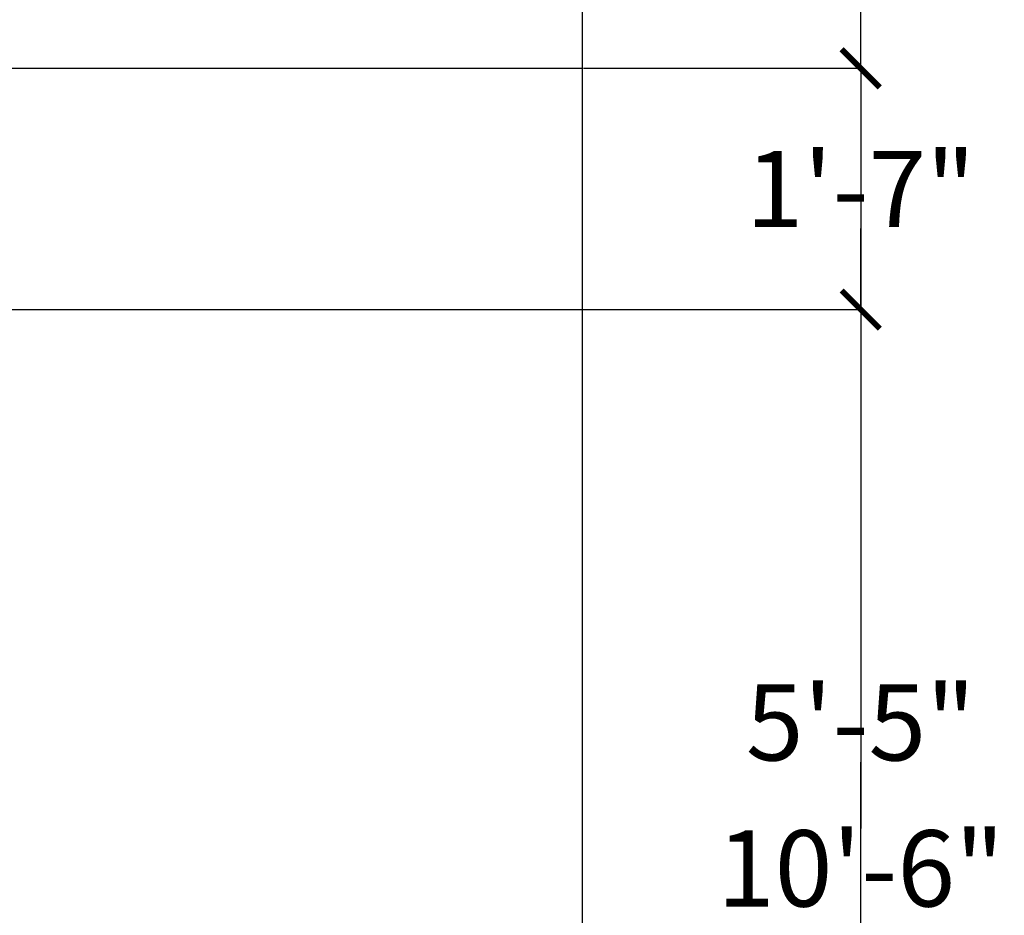
# Model space of a CAD drawing. Units: inches. Extents: x 2278 to 7495, y -71 to 1198.
# Tile 37 of 44: x 5101 to 5179, y 178 to 248. Entities that reach past the tile are written whole.
import ezdxf

# ---------------------------------------------------------------- set-up
doc = ezdxf.new("R2010")
doc.units = ezdxf.units.IN
doc.header["$MEASUREMENT"] = 0
doc.layers.add('A-ANNO-DIMS', color=2, linetype='Continuous', lineweight=18)
doc.layers.add('A-ELEV', color=7, linetype='Continuous', lineweight=25)
doc.styles.get("Standard").update_dxf_attribs({"font": 'arial.ttf'})
doc.dimstyles.get("Standard").update_dxf_attribs({"dimtxt": 6, "dimasz": 3, "dimexe": 0.18, "dimexo": 0.0625, "dimgap": 0.09, "dimtad": 0, "dimtih": 1, "dimtoh": 1, "dimdec": 0, "dimzin": 0, "dimdsep": 46, "dimlunit": 3, "dimtxsty": 'Standard', "dimblk": 'ARCHTICK', "dimcen": 0.09, "dimadec": 0, "dimazin": 0, "dimtfac": 1, "dimtdec": 0, "dimtofl": 0, "dimtmove": 0, "dimatfit": 3, "dimfxl": 1, "dimtolj": 1, "dimtzin": 0, "dimarcsym": 0})

# ---------------------------------------------------------------- blocks, each defined once
blk = doc.blocks.new('_ArchTick')
at = {"color": 0, "linetype": 'ByBlock', "const_width": 0.15}
blk.add_lwpolyline([(-0.5, -0.5), (0.5, 0.5)], dxfattribs=at)
blk = doc.blocks.new('*D123')
at = {"layer": 'A-ANNO-DIMS', "color": 0, "lineweight": -2, "transparency": 16777216}
for p, q in [((4736.95, 340.157), (4736.95, -23.427)), ((5145.676, -1.81), (5145.676, -23.427)), ((4736.95, -23.247), (4923.929, -23.247)), ((5145.676, -23.247), (4958.697, -23.247))]:
    blk.add_line(p, q, dxfattribs=at)
at = {"layer": 'Defpoints', "color": 0, "transparency": 16777216}
for p in [(4736.95, 340.219), (5145.676, -1.747), (5145.676, -23.247)]:
    blk.add_point(p, dxfattribs=at)
at = {"layer": 'A-ANNO-DIMS', "color": 0, "lineweight": -2, "transparency": 16777216, "xscale": 3, "yscale": 3, "zscale": 3, "rotation": 180}
blk.add_blockref('_ArchTick', (4736.95, -23.247), dxfattribs=at)
at = {"layer": 'A-ANNO-DIMS', "color": 0, "lineweight": -2, "transparency": 16777216, "xscale": 3, "yscale": 3, "zscale": 3}
blk.add_blockref('_ArchTick', (5145.676, -23.247), dxfattribs=at)
at = {"layer": 'A-ANNO-DIMS', "color": 0, "transparency": 16777216, "insert": (4941.313, -23.247), "char_height": 6, "attachment_point": 5}
blk.add_mtext('\\A1;34\'-0 1/2"', dxfattribs=at)
blk = doc.blocks.new('*D131')
at = {"layer": 'A-ANNO-DIMS', "color": 0, "lineweight": -2, "transparency": 16777216}
for p, q in [((5096.176, 99.315), (5096.176, 361.899)), ((5096.176, 361.719), (5105.75, 361.719)), ((5145.676, 361.719), (5136.102, 361.719)), ((5145.676, 118.315), (5145.676, 361.899))]:
    blk.add_line(p, q, dxfattribs=at)
at = {"layer": 'Defpoints', "color": 0, "transparency": 16777216}
for p in [(5145.676, 361.719), (5145.676, 118.253), (5096.176, 99.253)]:
    blk.add_point(p, dxfattribs=at)
at = {"layer": 'A-ANNO-DIMS', "color": 0, "lineweight": -2, "transparency": 16777216, "xscale": 3, "yscale": 3, "zscale": 3, "rotation": 180}
blk.add_blockref('_ArchTick', (5096.176, 361.719), dxfattribs=at)
at = {"layer": 'A-ANNO-DIMS', "color": 0, "lineweight": -2, "transparency": 16777216, "xscale": 3, "yscale": 3, "zscale": 3}
blk.add_blockref('_ArchTick', (5145.676, 361.719), dxfattribs=at)
at = {"layer": 'A-ANNO-DIMS', "color": 0, "transparency": 16777216, "insert": (5120.926, 361.719), "char_height": 6, "attachment_point": 5}
blk.add_mtext('\\A1;4\'-1 1/2"', dxfattribs=at)
blk = doc.blocks.new('*D140')
at = {"layer": 'A-ANNO-DIMS', "color": 0, "lineweight": -2, "transparency": 16777216}
for p, q in [((5096.239, 225.253), (5167.754, 225.253)), ((5167.574, 225.253), (5167.574, 195.894)), ((5167.574, 160.253), (5167.574, 189.612)), ((5092.239, 160.253), (5167.754, 160.253))]:
    blk.add_line(p, q, dxfattribs=at)
at = {"layer": 'Defpoints', "color": 0, "transparency": 16777216}
for p in [(5096.176, 225.253), (5167.574, 225.253), (5092.176, 160.253)]:
    blk.add_point(p, dxfattribs=at)
at = {"layer": 'A-ANNO-DIMS', "color": 0, "lineweight": -2, "transparency": 16777216, "xscale": 3, "yscale": 3, "zscale": 3}
for p, rotation in [((5167.574, 225.253), 90), ((5167.574, 160.253), 270)]:
    blk.add_blockref('_ArchTick', p, dxfattribs=dict(at, rotation=rotation))
at = {"layer": 'A-ANNO-DIMS', "color": 0, "transparency": 16777216, "insert": (5167.574, 192.753), "char_height": 6, "attachment_point": 5}
blk.add_mtext('\\A1;5\'-5"', dxfattribs=at)
blk = doc.blocks.new('*D141')
at = {"layer": 'A-ANNO-DIMS', "color": 0, "lineweight": -2, "transparency": 16777216}
for p, q in [((5145.739, 244.253), (5167.754, 244.253)), ((5167.574, 244.253), (5167.574, 237.855)), ((5167.574, 225.253), (5167.574, 231.651)), ((5096.239, 225.253), (5167.754, 225.253))]:
    blk.add_line(p, q, dxfattribs=at)
at = {"layer": 'Defpoints', "color": 0, "transparency": 16777216}
for p in [(5145.676, 244.253), (5167.574, 244.253), (5096.176, 225.253)]:
    blk.add_point(p, dxfattribs=at)
at = {"layer": 'A-ANNO-DIMS', "color": 0, "lineweight": -2, "transparency": 16777216, "xscale": 3, "yscale": 3, "zscale": 3}
for p, rotation in [((5167.574, 244.253), 90), ((5167.574, 225.253), 270)]:
    blk.add_blockref('_ArchTick', p, dxfattribs=dict(at, rotation=rotation))
at = {"layer": 'A-ANNO-DIMS', "color": 0, "transparency": 16777216, "insert": (5167.574, 234.753), "char_height": 6, "attachment_point": 5}
blk.add_mtext('\\A1;1\'-7"', dxfattribs=at)
blk = doc.blocks.new('*D142')
at = {"layer": 'A-ANNO-DIMS', "color": 0, "lineweight": -2, "transparency": 16777216}
for p, q in [((5143.335, 286.303), (5167.754, 286.303)), ((5167.574, 286.303), (5167.574, 268.433)), ((5167.574, 244.253), (5167.574, 262.122)), ((5145.739, 244.253), (5167.754, 244.253))]:
    blk.add_line(p, q, dxfattribs=at)
at = {"layer": 'Defpoints', "color": 0, "transparency": 16777216}
for p in [(5143.273, 286.303), (5167.574, 286.303), (5145.676, 244.253)]:
    blk.add_point(p, dxfattribs=at)
at = {"layer": 'A-ANNO-DIMS', "color": 0, "lineweight": -2, "transparency": 16777216, "xscale": 3, "yscale": 3, "zscale": 3}
for p, rotation in [((5167.574, 286.303), 90), ((5167.574, 244.253), 270)]:
    blk.add_blockref('_ArchTick', p, dxfattribs=dict(at, rotation=rotation))
at = {"layer": 'A-ANNO-DIMS', "color": 0, "transparency": 16777216, "insert": (5167.574, 265.278), "char_height": 6, "attachment_point": 5}
blk.add_mtext('\\A1;3\'-6"', dxfattribs=at)
blk = doc.blocks.new('*D144')
at = {"layer": 'A-ANNO-DIMS', "color": 0, "lineweight": -2, "transparency": 16777216}
for p, q in [((5145.739, 244.253), (5167.754, 244.253)), ((5167.574, 244.253), (5167.574, 184.406)), ((5167.574, 118.253), (5167.574, 178.099)), ((5145.739, 118.253), (5167.754, 118.253))]:
    blk.add_line(p, q, dxfattribs=at)
at = {"layer": 'Defpoints', "color": 0, "transparency": 16777216}
for p in [(5145.676, 244.253), (5167.574, 244.253), (5145.676, 118.253)]:
    blk.add_point(p, dxfattribs=at)
at = {"layer": 'A-ANNO-DIMS', "color": 0, "lineweight": -2, "transparency": 16777216, "xscale": 3, "yscale": 3, "zscale": 3}
for p, rotation in [((5167.574, 244.253), 90), ((5167.574, 118.253), 270)]:
    blk.add_blockref('_ArchTick', p, dxfattribs=dict(at, rotation=rotation))
at = {"layer": 'A-ANNO-DIMS', "color": 0, "transparency": 16777216, "insert": (5167.574, 181.253), "char_height": 6, "attachment_point": 5}
blk.add_mtext('\\A1;10\'-6"', dxfattribs=at)

msp = doc.modelspace()

# ---------------------------------------------------------------- linework, layer by layer
at = {"layer": 'A-ELEV'}
for p, q in [((5145.676, 164.446), (5145.676, 250.254)), ((4874.676, 244.253), (5145.676, 244.253))]:
    msp.add_line(p, q, dxfattribs=at)

# ---------------------------------------------------------------- dimensions: what is measured, and where the dimension line sits
at = {"layer": 'A-ANNO-DIMS'}
for base, p1, p2, picture, middle in [((5145.676, 361.719), (5096.176, 99.253), (5145.676, 118.253), '*D131', (5120.926, 361.719)), ((5145.676, -23.247), (4736.95, 340.219), (5145.676, -1.747), '*D123', (4941.313, -23.247))]:
    dim = msp.add_linear_dim(base=base, p1=p1, p2=p2, dimstyle='Standard', override={"dimdec": 1, "dimlfac": 1, "dimrnd": 0, "dimzin": 1, "dimdsep": 46, "dimlunit": 4, "dimfrac": 2}, dxfattribs=at)
    dim.commit()
    dim.dimension.update_dxf_attribs({"geometry": picture, "text_midpoint": middle})
for base, p1, p2, picture, middle in [((5167.5738, 286.3026), (5145.6762, 244.2528), (5143.2729, 286.3026), '*D142', (5167.5738, 265.2777)), ((5167.574, 244.253), (5096.176, 225.253), (5145.676, 244.253), '*D141', (5167.574, 234.753)), ((5167.574, 244.253), (5145.676, 118.253), (5145.676, 244.253), '*D144', (5167.574, 181.253)), ((5167.574, 225.253), (5092.176, 160.253), (5096.176, 225.253), '*D140', (5167.574, 192.753))]:
    dim = msp.add_linear_dim(base=base, p1=p1, p2=p2, angle=90, dimstyle='Standard', override={"dimdec": 1, "dimlfac": 1, "dimrnd": 0, "dimzin": 1, "dimdsep": 46, "dimlunit": 4, "dimfrac": 2}, dxfattribs=at)
    dim.commit()
    dim.dimension.update_dxf_attribs({"geometry": picture, "text_midpoint": middle})

doc.saveas('drawing.dxf')
